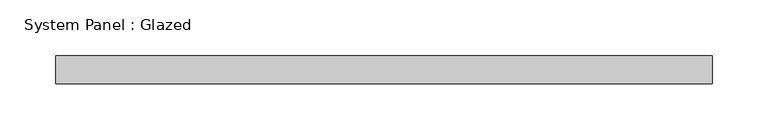
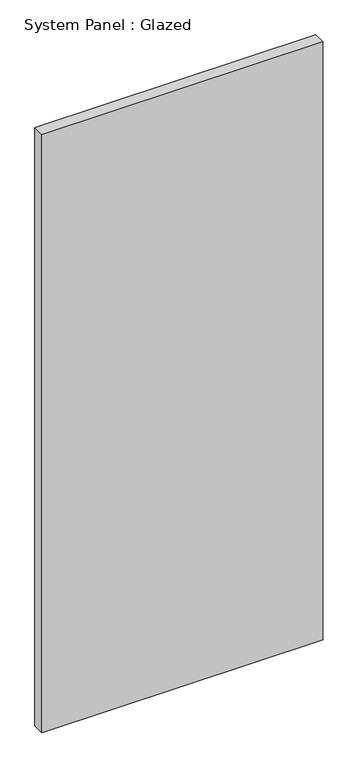
"""IFC4 building model written with IfcOpenShell, lengths in millimetres: plate geometry, System Panel : Glazed."""

from ifc_helpers import new_model, si_unit, origin, origin_with_axes, place, context, project, spatial, polyline, outline, extrude, source, transform, mapped, element, save


def system_panel_glazed_7c0c5eec(model_context):
    return source(origin(), model_context, "Body", "SweptSolid", [
        extrude(outline(polyline([(295.275, 19.05), (-295.275, 19.05), (-295.275, 44.45), (295.275, 44.45), (295.275, 19.05)])), origin_with_axes(), (0.0, 0.0, 1.0), 1329.6512079),
    ])


if __name__ == "__main__":
    model = new_model("IFC4")
    model_context = context("Model", 3, world=origin())
    ifc_project = project(units=[si_unit("LENGTHUNIT", "METRE", prefix="MILLI")], contexts=[model_context])
    site = spatial("IfcSite", under=ifc_project)
    building = spatial("IfcBuilding", under=site)
    placement = place(None, origin())
    system_panel_glazed_shape = system_panel_glazed_7c0c5eec(model_context)
    element("IfcPlate", 1, ObjectType="System Panel : Glazed", at=placement, inside=building, context=model_context, shape_type="MappedRepresentation", body=[
        mapped(system_panel_glazed_shape, transform((0.0, 0.0, 0.0), x_axis=(1.0, 0.0, 0.0), y_axis=(0.0, 1.0, 0.0), z_axis=(0.0, 0.0, 1.0))),
    ])
    save(model, "model.ifc")

# Revit data of these elements
# Type "System Panel : Glazed"
#   Construction Type Id = "GSP4R"
#   Analytic Construction = "1/8 in Pilkington single glazing"
#   Visual Light Transmittance = 0.9
#   Solar Heat Gain Coefficient = 0.86
#   Heat Transfer Coefficient (U) = 1.18115 BTU/(h·ft²·°F)
#   Define Thermal Properties by = 1
# Element 1 (IfcPlate, "System Panel : Glazed")
#   Materials on its faces: "Glass"
# Materials
#   "Glass": class "Glass", colour RGB 0 128 192, transparency 0.75, Description = "Soda Lime Glass", Cost = 0
